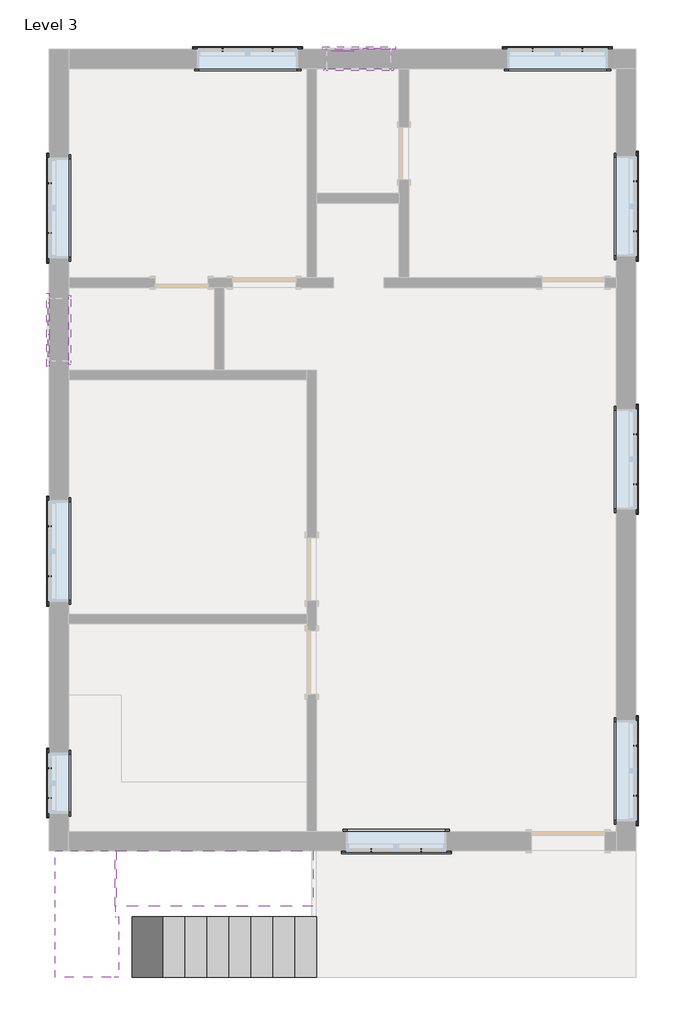
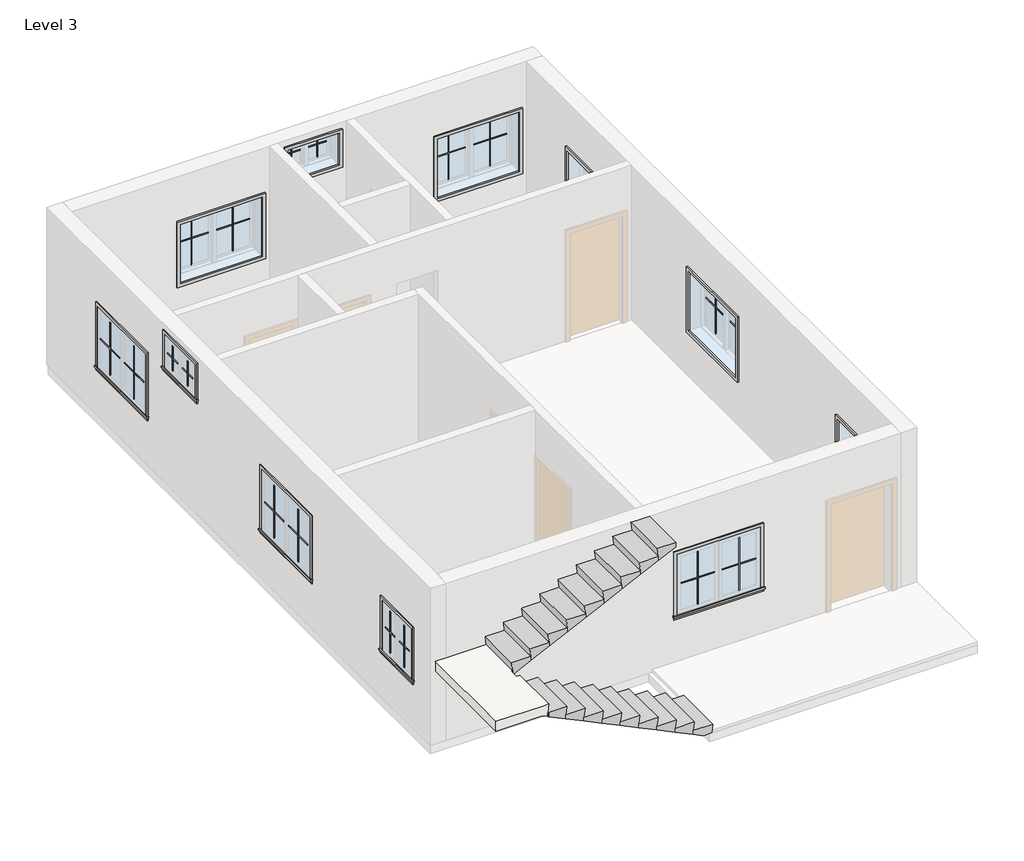
# One storey, part 2 of 2: 44 proxies, 2 stair flights, 1 slab.
"""IFC4 building model written with IfcOpenShell, lengths in millimetres."""

from ifc_helpers import new_model, si_unit, origin, place, context, project, spatial, faceted_brep, transform, mapped, element, save
from components import muntin_pattern_2x2_muntin_pattern_2x2_b3fe6957, muntin_pattern_2x2_muntin_pattern_2x2_3e0ecaf2, muntin_pattern_2x2_muntin_pattern_2x2_27d56209, muntin_pattern_2x2_muntin_pattern_2x2_bc89accc, muntin_pattern_2x2_muntin_pattern_2x2_1fe271a4, muntin_pattern_2x2_muntin_pattern_2x2_11ff06db, trim_window_exterior_flat_with_sill_41619996, trim_window_exterior_flat_with_sill_40e754a6, trim_window_exterior_flat_with_sill_f4abd27b, trim_window_interior_flat_picture_frame_51c85655, trim_window_interior_flat_picture_frame_6592d821, trim_window_interior_flat_picture_frame_286514af

model = new_model("IFC4")

# Units and contexts
model_context = context("Model", 3, world=origin())
ifc_project = project(units=[si_unit("LENGTHUNIT", "METRE", prefix="MILLI")], contexts=[model_context])

# Site, building, storey
site = spatial("IfcSite", under=ifc_project)
building = spatial("IfcBuilding", under=site)
storey = spatial("IfcBuildingStorey", under=building, Name="Level 3", Elevation=6096.0)

# Proxies
placement = place(None, origin())
muntin_pattern_2x2_muntin_pattern_2x2_shape = muntin_pattern_2x2_muntin_pattern_2x2_b3fe6957(model_context)
element("IfcBuildingElementProxy", 1, Name="Muntin Pattern_2x2 : Muntin Pattern_2x2", ObjectType="Muntin Pattern_2x2 : Muntin Pattern_2x2", at=placement, inside=storey, context=model_context, shape_type="MappedRepresentation", body=[
    mapped(muntin_pattern_2x2_muntin_pattern_2x2_shape, transform((-8839.6634077, -4303.4328663, 7080.25), x_axis=(0.0, 1.0, 0.0), y_axis=(-1.0, 0.0, 0.0), z_axis=(0.0, 0.0, 1.0))),
])
muntin_pattern_2x2_muntin_pattern_2x2_2_shape = muntin_pattern_2x2_muntin_pattern_2x2_3e0ecaf2(model_context)
element("IfcBuildingElementProxy", 2, Name="Muntin Pattern_2x2 : Muntin Pattern_2x2", ObjectType="Muntin Pattern_2x2 : Muntin Pattern_2x2", at=placement, inside=storey, context=model_context, shape_type="MappedRepresentation", body=[
    mapped(muntin_pattern_2x2_muntin_pattern_2x2_2_shape, transform((-8839.6634077, -3874.8078663, 7080.25), x_axis=(0.0, -1.0, 0.0), y_axis=(1.0, 0.0, 0.0), z_axis=(0.0, 0.0, 1.0))),
])
muntin_pattern_2x2_muntin_pattern_2x2_3_shape = muntin_pattern_2x2_muntin_pattern_2x2_27d56209(model_context)
element("IfcBuildingElementProxy", 3, Name="Muntin Pattern_2x2 : Muntin Pattern_2x2", ObjectType="Muntin Pattern_2x2 : Muntin Pattern_2x2", at=placement, inside=storey, context=model_context, shape_type="MappedRepresentation", body=[
    mapped(muntin_pattern_2x2_muntin_pattern_2x2_3_shape, transform((-8839.6634077, 2226.7657273, 8299.45), x_axis=(0.0, 1.0, 0.0), y_axis=(-1.0, 0.0, 0.0), z_axis=(0.0, 0.0, 1.0))),
])
element("IfcBuildingElementProxy", 4, Name="Muntin Pattern_2x2 : Muntin Pattern_2x2", ObjectType="Muntin Pattern_2x2 : Muntin Pattern_2x2", at=placement, inside=storey, context=model_context, shape_type="MappedRepresentation", body=[
    mapped(muntin_pattern_2x2_muntin_pattern_2x2_3_shape, transform((-4603.9220229, 6494.5392844, 8299.45), x_axis=(1.0, 0.0, 0.0), y_axis=(0.0, 1.0, 0.0), z_axis=(0.0, 0.0, 1.0))),
])
muntin_pattern_2x2_muntin_pattern_2x2_4_shape = muntin_pattern_2x2_muntin_pattern_2x2_bc89accc(model_context)
element("IfcBuildingElementProxy", 5, Name="Muntin Pattern_2x2 : Muntin Pattern_2x2", ObjectType="Muntin Pattern_2x2 : Muntin Pattern_2x2", at=placement, inside=storey, context=model_context, shape_type="MappedRepresentation", body=[
    mapped(muntin_pattern_2x2_muntin_pattern_2x2_4_shape, transform((-8839.6634077, 2680.7907273, 8299.45), x_axis=(0.0, -1.0, 0.0), y_axis=(1.0, 0.0, 0.0), z_axis=(0.0, 0.0, 1.0))),
])
element("IfcBuildingElementProxy", 6, Name="Muntin Pattern_2x2 : Muntin Pattern_2x2", ObjectType="Muntin Pattern_2x2 : Muntin Pattern_2x2", at=placement, inside=storey, context=model_context, shape_type="MappedRepresentation", body=[
    mapped(muntin_pattern_2x2_muntin_pattern_2x2_4_shape, transform((-4149.8970229, 6494.5392844, 8299.45), x_axis=(-1.0, 0.0, 0.0), y_axis=(0.0, -1.0, 0.0), z_axis=(0.0, 0.0, 1.0))),
])
muntin_pattern_2x2_muntin_pattern_2x2_5_shape = muntin_pattern_2x2_muntin_pattern_2x2_1fe271a4(model_context)
element("IfcBuildingElementProxy", 7, Name="Muntin Pattern_2x2 : Muntin Pattern_2x2", ObjectType="Muntin Pattern_2x2 : Muntin Pattern_2x2", at=placement, inside=storey, context=model_context, shape_type="MappedRepresentation", body=[
    mapped(muntin_pattern_2x2_muntin_pattern_2x2_5_shape, transform((-385.3035282, -3550.9578663, 7080.25), x_axis=(0.0, -1.0, 0.0), y_axis=(1.0, 0.0, 0.0), z_axis=(0.0, 0.0, 1.0))),
])
element("IfcBuildingElementProxy", 8, Name="Muntin Pattern_2x2 : Muntin Pattern_2x2", ObjectType="Muntin Pattern_2x2 : Muntin Pattern_2x2", at=placement, inside=storey, context=model_context, shape_type="MappedRepresentation", body=[
    mapped(muntin_pattern_2x2_muntin_pattern_2x2_5_shape, transform((-385.3035282, 944.8421337, 7080.25), x_axis=(0.0, -1.0, 0.0), y_axis=(1.0, 0.0, 0.0), z_axis=(0.0, 0.0, 1.0))),
])
element("IfcBuildingElementProxy", 9, Name="Muntin Pattern_2x2 : Muntin Pattern_2x2", ObjectType="Muntin Pattern_2x2 : Muntin Pattern_2x2", at=placement, inside=storey, context=model_context, shape_type="MappedRepresentation", body=[
    mapped(muntin_pattern_2x2_muntin_pattern_2x2_5_shape, transform((-385.3035282, 4597.1928819, 7080.25), x_axis=(0.0, -1.0, 0.0), y_axis=(1.0, 0.0, 0.0), z_axis=(0.0, 0.0, 1.0))),
])
element("IfcBuildingElementProxy", 10, Name="Muntin Pattern_2x2 : Muntin Pattern_2x2", ObjectType="Muntin Pattern_2x2 : Muntin Pattern_2x2", at=placement, inside=storey, context=model_context, shape_type="MappedRepresentation", body=[
    mapped(muntin_pattern_2x2_muntin_pattern_2x2_5_shape, transform((-1866.4410282, 6494.5392844, 7080.25), x_axis=(1.0, 0.0, 0.0), y_axis=(0.0, 1.0, 0.0), z_axis=(0.0, 0.0, 1.0))),
])
element("IfcBuildingElementProxy", 11, Name="Muntin Pattern_2x2 : Muntin Pattern_2x2", ObjectType="Muntin Pattern_2x2 : Muntin Pattern_2x2", at=placement, inside=storey, context=model_context, shape_type="MappedRepresentation", body=[
    mapped(muntin_pattern_2x2_muntin_pattern_2x2_5_shape, transform((-6342.5074828, 6494.5392844, 7080.25), x_axis=(1.0, 0.0, 0.0), y_axis=(0.0, 1.0, 0.0), z_axis=(0.0, 0.0, 1.0))),
])
element("IfcBuildingElementProxy", 12, Name="Muntin Pattern_2x2 : Muntin Pattern_2x2", ObjectType="Muntin Pattern_2x2 : Muntin Pattern_2x2", at=placement, inside=storey, context=model_context, shape_type="MappedRepresentation", body=[
    mapped(muntin_pattern_2x2_muntin_pattern_2x2_5_shape, transform((-8839.6634077, 3851.0678819, 7080.25), x_axis=(0.0, 1.0, 0.0), y_axis=(-1.0, 0.0, 0.0), z_axis=(0.0, 0.0, 1.0))),
])
element("IfcBuildingElementProxy", 13, Name="Muntin Pattern_2x2 : Muntin Pattern_2x2", ObjectType="Muntin Pattern_2x2 : Muntin Pattern_2x2", at=placement, inside=storey, context=model_context, shape_type="MappedRepresentation", body=[
    mapped(muntin_pattern_2x2_muntin_pattern_2x2_5_shape, transform((-8839.6634077, -1101.0873314, 7080.25), x_axis=(0.0, 1.0, 0.0), y_axis=(-1.0, 0.0, 0.0), z_axis=(0.0, 0.0, 1.0))),
])
element("IfcBuildingElementProxy", 14, Name="Muntin Pattern_2x2 : Muntin Pattern_2x2", ObjectType="Muntin Pattern_2x2 : Muntin Pattern_2x2", at=placement, inside=storey, context=model_context, shape_type="MappedRepresentation", body=[
    mapped(muntin_pattern_2x2_muntin_pattern_2x2_5_shape, transform((-3475.4824828, -5057.4953663, 7080.25), x_axis=(-1.0, 0.0, 0.0), y_axis=(0.0, -1.0, 0.0), z_axis=(0.0, 0.0, 1.0))),
])
muntin_pattern_2x2_muntin_pattern_2x2_6_shape = muntin_pattern_2x2_muntin_pattern_2x2_11ff06db(model_context)
element("IfcBuildingElementProxy", 15, Name="Muntin Pattern_2x2 : Muntin Pattern_2x2", ObjectType="Muntin Pattern_2x2 : Muntin Pattern_2x2", at=placement, inside=storey, context=model_context, shape_type="MappedRepresentation", body=[
    mapped(muntin_pattern_2x2_muntin_pattern_2x2_6_shape, transform((-385.3035282, -4271.6828663, 7080.25), x_axis=(0.0, 1.0, 0.0), y_axis=(-1.0, 0.0, 0.0), z_axis=(0.0, 0.0, 1.0))),
])
element("IfcBuildingElementProxy", 16, Name="Muntin Pattern_2x2 : Muntin Pattern_2x2", ObjectType="Muntin Pattern_2x2 : Muntin Pattern_2x2", at=placement, inside=storey, context=model_context, shape_type="MappedRepresentation", body=[
    mapped(muntin_pattern_2x2_muntin_pattern_2x2_6_shape, transform((-385.3035282, 224.1171337, 7080.25), x_axis=(0.0, 1.0, 0.0), y_axis=(-1.0, 0.0, 0.0), z_axis=(0.0, 0.0, 1.0))),
])
element("IfcBuildingElementProxy", 17, Name="Muntin Pattern_2x2 : Muntin Pattern_2x2", ObjectType="Muntin Pattern_2x2 : Muntin Pattern_2x2", at=placement, inside=storey, context=model_context, shape_type="MappedRepresentation", body=[
    mapped(muntin_pattern_2x2_muntin_pattern_2x2_6_shape, transform((-385.3035282, 3876.4678819, 7080.25), x_axis=(0.0, 1.0, 0.0), y_axis=(-1.0, 0.0, 0.0), z_axis=(0.0, 0.0, 1.0))),
])
element("IfcBuildingElementProxy", 18, Name="Muntin Pattern_2x2 : Muntin Pattern_2x2", ObjectType="Muntin Pattern_2x2 : Muntin Pattern_2x2", at=placement, inside=storey, context=model_context, shape_type="MappedRepresentation", body=[
    mapped(muntin_pattern_2x2_muntin_pattern_2x2_6_shape, transform((-1145.7160282, 6494.5392844, 7080.25), x_axis=(-1.0, 0.0, 0.0), y_axis=(0.0, -1.0, 0.0), z_axis=(0.0, 0.0, 1.0))),
])
element("IfcBuildingElementProxy", 19, Name="Muntin Pattern_2x2 : Muntin Pattern_2x2", ObjectType="Muntin Pattern_2x2 : Muntin Pattern_2x2", at=placement, inside=storey, context=model_context, shape_type="MappedRepresentation", body=[
    mapped(muntin_pattern_2x2_muntin_pattern_2x2_6_shape, transform((-5621.7824828, 6494.5392844, 7080.25), x_axis=(-1.0, 0.0, 0.0), y_axis=(0.0, -1.0, 0.0), z_axis=(0.0, 0.0, 1.0))),
])
element("IfcBuildingElementProxy", 20, Name="Muntin Pattern_2x2 : Muntin Pattern_2x2", ObjectType="Muntin Pattern_2x2 : Muntin Pattern_2x2", at=placement, inside=storey, context=model_context, shape_type="MappedRepresentation", body=[
    mapped(muntin_pattern_2x2_muntin_pattern_2x2_6_shape, transform((-8839.6634077, 4571.7928819, 7080.25), x_axis=(0.0, -1.0, 0.0), y_axis=(1.0, 0.0, 0.0), z_axis=(0.0, 0.0, 1.0))),
])
element("IfcBuildingElementProxy", 21, Name="Muntin Pattern_2x2 : Muntin Pattern_2x2", ObjectType="Muntin Pattern_2x2 : Muntin Pattern_2x2", at=placement, inside=storey, context=model_context, shape_type="MappedRepresentation", body=[
    mapped(muntin_pattern_2x2_muntin_pattern_2x2_6_shape, transform((-8839.6634077, -380.3623314, 7080.25), x_axis=(0.0, -1.0, 0.0), y_axis=(1.0, 0.0, 0.0), z_axis=(0.0, 0.0, 1.0))),
])
element("IfcBuildingElementProxy", 22, Name="Muntin Pattern_2x2 : Muntin Pattern_2x2", ObjectType="Muntin Pattern_2x2 : Muntin Pattern_2x2", at=placement, inside=storey, context=model_context, shape_type="MappedRepresentation", body=[
    mapped(muntin_pattern_2x2_muntin_pattern_2x2_6_shape, transform((-4196.2074828, -5057.4953663, 7080.25), x_axis=(1.0, 0.0, 0.0), y_axis=(0.0, 1.0, 0.0), z_axis=(0.0, 0.0, 1.0))),
])
trim_window_exterior_flat_with_sill_shape = trim_window_exterior_flat_with_sill_41619996(model_context)
element("IfcBuildingElementProxy", 23, Name="Trim-Window-Exterior-Flat : with Sill", ObjectType="Trim-Window-Exterior-Flat : with Sill", at=placement, inside=storey, context=model_context, shape_type="MappedRepresentation", body=[
    mapped(trim_window_exterior_flat_with_sill_shape, transform((-8849.1884077, -4089.1203663, 7924.8), x_axis=(0.0, -1.0, 0.0), y_axis=(0.0, 0.0, 1.0), z_axis=(-1.0, 0.0, 0.0))),
])
trim_window_exterior_flat_with_sill_2_shape = trim_window_exterior_flat_with_sill_40e754a6(model_context)
element("IfcBuildingElementProxy", 24, Name="Trim-Window-Exterior-Flat : with Sill", ObjectType="Trim-Window-Exterior-Flat : with Sill", at=placement, inside=storey, context=model_context, shape_type="MappedRepresentation", body=[
    mapped(trim_window_exterior_flat_with_sill_2_shape, transform((-8849.1884077, 2453.7782273, 8839.2), x_axis=(0.0, -1.0, 0.0), y_axis=(0.0, 0.0, 1.0), z_axis=(-1.0, 0.0, 0.0))),
])
element("IfcBuildingElementProxy", 25, Name="Trim-Window-Exterior-Flat : with Sill", ObjectType="Trim-Window-Exterior-Flat : with Sill", at=placement, inside=storey, context=model_context, shape_type="MappedRepresentation", body=[
    mapped(trim_window_exterior_flat_with_sill_2_shape, transform((-4376.9095229, 6504.0642844, 8839.2), x_axis=(-1.0, 0.0, 0.0), y_axis=(0.0, 0.0, 1.0), z_axis=(0.0, 1.0, 0.0))),
])
trim_window_exterior_flat_with_sill_3_shape = trim_window_exterior_flat_with_sill_f4abd27b(model_context)
element("IfcBuildingElementProxy", 26, Name="Trim-Window-Exterior-Flat : with Sill", ObjectType="Trim-Window-Exterior-Flat : with Sill", at=placement, inside=storey, context=model_context, shape_type="MappedRepresentation", body=[
    mapped(trim_window_exterior_flat_with_sill_3_shape, transform((-375.7785282, -3911.3203663, 8128.0), x_axis=(0.0, 1.0, 0.0), y_axis=(0.0, 0.0, 1.0), z_axis=(1.0, 0.0, 0.0))),
])
element("IfcBuildingElementProxy", 27, Name="Trim-Window-Exterior-Flat : with Sill", ObjectType="Trim-Window-Exterior-Flat : with Sill", at=placement, inside=storey, context=model_context, shape_type="MappedRepresentation", body=[
    mapped(trim_window_exterior_flat_with_sill_3_shape, transform((-375.7785282, 584.4796337, 8128.0), x_axis=(0.0, 1.0, 0.0), y_axis=(0.0, 0.0, 1.0), z_axis=(1.0, 0.0, 0.0))),
])
element("IfcBuildingElementProxy", 28, Name="Trim-Window-Exterior-Flat : with Sill", ObjectType="Trim-Window-Exterior-Flat : with Sill", at=placement, inside=storey, context=model_context, shape_type="MappedRepresentation", body=[
    mapped(trim_window_exterior_flat_with_sill_3_shape, transform((-375.7785282, 4236.8303819, 8128.0), x_axis=(0.0, 1.0, 0.0), y_axis=(0.0, 0.0, 1.0), z_axis=(1.0, 0.0, 0.0))),
])
element("IfcBuildingElementProxy", 29, Name="Trim-Window-Exterior-Flat : with Sill", ObjectType="Trim-Window-Exterior-Flat : with Sill", at=placement, inside=storey, context=model_context, shape_type="MappedRepresentation", body=[
    mapped(trim_window_exterior_flat_with_sill_3_shape, transform((-1506.0785282, 6504.0642844, 8128.0), x_axis=(-1.0, 0.0, 0.0), y_axis=(0.0, 0.0, 1.0), z_axis=(0.0, 1.0, 0.0))),
])
element("IfcBuildingElementProxy", 30, Name="Trim-Window-Exterior-Flat : with Sill", ObjectType="Trim-Window-Exterior-Flat : with Sill", at=placement, inside=storey, context=model_context, shape_type="MappedRepresentation", body=[
    mapped(trim_window_exterior_flat_with_sill_3_shape, transform((-5982.1449828, 6504.0642844, 8128.0), x_axis=(-1.0, 0.0, 0.0), y_axis=(0.0, 0.0, 1.0), z_axis=(0.0, 1.0, 0.0))),
])
element("IfcBuildingElementProxy", 31, Name="Trim-Window-Exterior-Flat : with Sill", ObjectType="Trim-Window-Exterior-Flat : with Sill", at=placement, inside=storey, context=model_context, shape_type="MappedRepresentation", body=[
    mapped(trim_window_exterior_flat_with_sill_3_shape, transform((-8849.1884077, 4211.4303819, 8128.0), x_axis=(0.0, -1.0, 0.0), y_axis=(0.0, 0.0, 1.0), z_axis=(-1.0, 0.0, 0.0))),
])
element("IfcBuildingElementProxy", 32, Name="Trim-Window-Exterior-Flat : with Sill", ObjectType="Trim-Window-Exterior-Flat : with Sill", at=placement, inside=storey, context=model_context, shape_type="MappedRepresentation", body=[
    mapped(trim_window_exterior_flat_with_sill_3_shape, transform((-8849.1884077, -740.7248314, 8128.0), x_axis=(0.0, -1.0, 0.0), y_axis=(0.0, 0.0, 1.0), z_axis=(-1.0, 0.0, 0.0))),
])
element("IfcBuildingElementProxy", 33, Name="Trim-Window-Exterior-Flat : with Sill", ObjectType="Trim-Window-Exterior-Flat : with Sill", at=placement, inside=storey, context=model_context, shape_type="MappedRepresentation", body=[
    mapped(trim_window_exterior_flat_with_sill_3_shape, transform((-3835.8449828, -5067.0203663, 8128.0), x_axis=(1.0, 0.0, 0.0), y_axis=(0.0, 0.0, 1.0), z_axis=(0.0, -1.0, 0.0))),
])
trim_window_interior_flat_picture_frame_shape = trim_window_interior_flat_picture_frame_51c85655(model_context)
element("IfcBuildingElementProxy", 34, Name="Trim-Window-Interior-Flat : Picture Frame", ObjectType="Trim-Window-Interior-Flat : Picture Frame", at=placement, inside=storey, context=model_context, shape_type="MappedRepresentation", body=[
    mapped(trim_window_interior_flat_picture_frame_shape, transform((-8569.7884077, -4089.1203663, 7924.8), x_axis=(0.0, 1.0, 0.0), y_axis=(0.0, 0.0, 1.0), z_axis=(1.0, 0.0, 0.0))),
])
trim_window_interior_flat_picture_frame_2_shape = trim_window_interior_flat_picture_frame_6592d821(model_context)
element("IfcBuildingElementProxy", 35, Name="Trim-Window-Interior-Flat : Picture Frame", ObjectType="Trim-Window-Interior-Flat : Picture Frame", at=placement, inside=storey, context=model_context, shape_type="MappedRepresentation", body=[
    mapped(trim_window_interior_flat_picture_frame_2_shape, transform((-8569.7884077, 2453.7782273, 8839.2), x_axis=(0.0, 1.0, 0.0), y_axis=(0.0, 0.0, 1.0), z_axis=(1.0, 0.0, 0.0))),
])
element("IfcBuildingElementProxy", 36, Name="Trim-Window-Interior-Flat : Picture Frame", ObjectType="Trim-Window-Interior-Flat : Picture Frame", at=placement, inside=storey, context=model_context, shape_type="MappedRepresentation", body=[
    mapped(trim_window_interior_flat_picture_frame_2_shape, transform((-4376.9095229, 6224.6642844, 8839.2), x_axis=(1.0, 0.0, 0.0), y_axis=(0.0, 0.0, 1.0), z_axis=(0.0, -1.0, 0.0))),
])
trim_window_interior_flat_picture_frame_3_shape = trim_window_interior_flat_picture_frame_286514af(model_context)
element("IfcBuildingElementProxy", 37, Name="Trim-Window-Interior-Flat : Picture Frame", ObjectType="Trim-Window-Interior-Flat : Picture Frame", at=placement, inside=storey, context=model_context, shape_type="MappedRepresentation", body=[
    mapped(trim_window_interior_flat_picture_frame_3_shape, transform((-655.1785282, -3911.3203663, 8128.0), x_axis=(0.0, -1.0, 0.0), y_axis=(0.0, 0.0, 1.0), z_axis=(-1.0, 0.0, 0.0))),
])
element("IfcBuildingElementProxy", 38, Name="Trim-Window-Interior-Flat : Picture Frame", ObjectType="Trim-Window-Interior-Flat : Picture Frame", at=placement, inside=storey, context=model_context, shape_type="MappedRepresentation", body=[
    mapped(trim_window_interior_flat_picture_frame_3_shape, transform((-655.1785282, 584.4796337, 8128.0), x_axis=(0.0, -1.0, 0.0), y_axis=(0.0, 0.0, 1.0), z_axis=(-1.0, 0.0, 0.0))),
])
element("IfcBuildingElementProxy", 39, Name="Trim-Window-Interior-Flat : Picture Frame", ObjectType="Trim-Window-Interior-Flat : Picture Frame", at=placement, inside=storey, context=model_context, shape_type="MappedRepresentation", body=[
    mapped(trim_window_interior_flat_picture_frame_3_shape, transform((-655.1785282, 4236.8303819, 8128.0), x_axis=(0.0, -1.0, 0.0), y_axis=(0.0, 0.0, 1.0), z_axis=(-1.0, 0.0, 0.0))),
])
element("IfcBuildingElementProxy", 40, Name="Trim-Window-Interior-Flat : Picture Frame", ObjectType="Trim-Window-Interior-Flat : Picture Frame", at=placement, inside=storey, context=model_context, shape_type="MappedRepresentation", body=[
    mapped(trim_window_interior_flat_picture_frame_3_shape, transform((-1506.0785282, 6224.6642844, 8128.0), x_axis=(1.0, 0.0, 0.0), y_axis=(0.0, 0.0, 1.0), z_axis=(0.0, -1.0, 0.0))),
])
element("IfcBuildingElementProxy", 41, Name="Trim-Window-Interior-Flat : Picture Frame", ObjectType="Trim-Window-Interior-Flat : Picture Frame", at=placement, inside=storey, context=model_context, shape_type="MappedRepresentation", body=[
    mapped(trim_window_interior_flat_picture_frame_3_shape, transform((-5982.1449828, 6224.6642844, 8128.0), x_axis=(1.0, 0.0, 0.0), y_axis=(0.0, 0.0, 1.0), z_axis=(0.0, -1.0, 0.0))),
])
element("IfcBuildingElementProxy", 42, Name="Trim-Window-Interior-Flat : Picture Frame", ObjectType="Trim-Window-Interior-Flat : Picture Frame", at=placement, inside=storey, context=model_context, shape_type="MappedRepresentation", body=[
    mapped(trim_window_interior_flat_picture_frame_3_shape, transform((-8569.7884077, 4211.4303819, 8128.0), x_axis=(0.0, 1.0, 0.0), y_axis=(0.0, 0.0, 1.0), z_axis=(1.0, 0.0, 0.0))),
])
element("IfcBuildingElementProxy", 43, Name="Trim-Window-Interior-Flat : Picture Frame", ObjectType="Trim-Window-Interior-Flat : Picture Frame", at=placement, inside=storey, context=model_context, shape_type="MappedRepresentation", body=[
    mapped(trim_window_interior_flat_picture_frame_3_shape, transform((-8569.7884077, -740.7248314, 8128.0), x_axis=(0.0, 1.0, 0.0), y_axis=(0.0, 0.0, 1.0), z_axis=(1.0, 0.0, 0.0))),
])
element("IfcBuildingElementProxy", 44, Name="Trim-Window-Interior-Flat : Picture Frame", ObjectType="Trim-Window-Interior-Flat : Picture Frame", at=placement, inside=storey, context=model_context, shape_type="MappedRepresentation", body=[
    mapped(trim_window_interior_flat_picture_frame_3_shape, transform((-3835.8449828, -4787.6203663, 8128.0), x_axis=(-1.0, 0.0, 0.0), y_axis=(0.0, 0.0, 1.0), z_axis=(0.0, 1.0, 0.0))),
])

# Slab
element("IfcSlab", 45, ObjectType="7\" Thickness", at=placement, inside=storey, context=model_context, shape_type="Brep", body=[
    faceted_brep([(-7896.6884077, -6018.2039507, 7620.0), (-7896.6884077, -5868.2058051, 7620.0), (-7877.6384077, -5868.2058051, 7620.0), (-7877.6384077, -5067.0203663, 7620.0), (-7896.6884077, -5067.0203663, 7620.0), (-8101.3126638, -5067.0203663, 7620.0), (-8760.2884077, -5067.0203663, 7620.0), (-8760.2884077, -6894.0922127, 7620.0), (-7955.5707267, -6894.0922127, 7620.0), (-7842.6949828, -6894.0922127, 7620.0), (-7842.6949828, -6018.2039507, 7620.0), (-7861.7449828, -6018.2039507, 7467.6), (-7861.7449828, -6894.0922127, 7467.6), (-7861.7449828, -6894.0922127, 7397.1636429), (-7861.7449828, -6018.2039507, 7397.1636429), (-7955.5707267, -6018.2039507, 7442.2), (-7896.6884077, -6018.2039507, 7442.2), (-7896.6884077, -5868.2058051, 7442.2), (-7896.6884077, -5868.2058051, 7540.4196429), (-7877.6384077, -5868.2058051, 7549.5636429), (-7877.6384077, -5067.0203663, 7549.5636429), (-7896.6884077, -5067.0203663, 7540.4196429), (-8101.3126638, -5067.0203663, 7442.2), (-8760.2884077, -5067.0203663, 7442.2), (-8760.2884077, -6894.0922127, 7442.2), (-7955.5707267, -6894.0922127, 7442.2), (-8101.3126638, -5868.2058051, 7442.2)], [[[0, 1, 2, 3, 4, 5, 6, 7, 8, 9, 10]], [[11, 12, 13, 14]], [[0, 10, 11, 14, 15, 16]], [[1, 0, 16, 17, 18]], [[2, 1, 18, 19]], [[3, 2, 19, 20]], [[4, 3, 20, 21]], [[4, 21, 22, 23, 6, 5]], [[7, 6, 23, 24]], [[12, 9, 8, 7, 24, 25, 13]], [[10, 9, 12, 11]], [[26, 17, 16, 15, 25, 24, 23, 22]], [[17, 26, 18]], [[25, 15, 14, 13]], [[26, 22, 21, 20, 19, 18]]]),
])

# Stair flights
element("IfcStairFlight", 46, ObjectType="3/4\" Nosing", at=placement, inside=storey, context=model_context, shape_type="Brep", body=[
    faceted_brep([(-4985.1949828, -6894.0922127, 6248.4), (-4985.1949828, -6018.2039507, 6248.4), (-5321.7449828, -6018.2039507, 6248.4), (-5321.7449828, -6894.0922127, 6248.4), (-5321.7449828, -6894.0922127, 6177.9636429), (-5150.9873934, -6894.0922127, 6096.0), (-5004.2449828, -6894.0922127, 6096.0), (-5004.2449828, -6018.2039507, 6096.0), (-5150.9873934, -6018.2039507, 6096.0), (-5321.7449828, -6018.2039507, 6177.9636429), (-5302.6949828, -6894.0922127, 6400.8), (-5302.6949828, -6018.2039507, 6400.8), (-5639.2449828, -6018.2039507, 6400.8), (-5639.2449828, -6894.0922127, 6400.8), (-5639.2449828, -6894.0922127, 6330.3636429), (-5639.2449828, -6018.2039507, 6330.3636429), (-5620.1949828, -6894.0922127, 6553.2), (-5620.1949828, -6018.2039507, 6553.2), (-5956.7449828, -6018.2039507, 6553.2), (-5956.7449828, -6894.0922127, 6553.2), (-5956.7449828, -6894.0922127, 6482.7636429), (-5956.7449828, -6018.2039507, 6482.7636429), (-5937.6949828, -6894.0922127, 6705.6), (-5937.6949828, -6018.2039507, 6705.6), (-6274.2449828, -6018.2039507, 6705.6), (-6274.2449828, -6894.0922127, 6705.6), (-6274.2449828, -6894.0922127, 6635.1636429), (-6274.2449828, -6018.2039507, 6635.1636429), (-6255.1949828, -6894.0922127, 6858.0), (-6255.1949828, -6018.2039507, 6858.0), (-6591.7449828, -6018.2039507, 6858.0), (-6591.7449828, -6894.0922127, 6858.0), (-6591.7449828, -6894.0922127, 6787.5636429), (-6591.7449828, -6018.2039507, 6787.5636429), (-6572.6949828, -6894.0922127, 7010.4), (-6572.6949828, -6018.2039507, 7010.4), (-6909.2449828, -6018.2039507, 7010.4), (-6909.2449828, -6894.0922127, 7010.4), (-6909.2449828, -6894.0922127, 6939.9636429), (-6909.2449828, -6018.2039507, 6939.9636429), (-6890.1949828, -6894.0922127, 7162.8), (-6890.1949828, -6018.2039507, 7162.8), (-7226.7449828, -6018.2039507, 7162.8), (-7226.7449828, -6894.0922127, 7162.8), (-7226.7449828, -6894.0922127, 7092.3636429), (-7226.7449828, -6018.2039507, 7092.3636429), (-7207.6949828, -6894.0922127, 7315.2), (-7207.6949828, -6018.2039507, 7315.2), (-7544.2449828, -6018.2039507, 7315.2), (-7544.2449828, -6894.0922127, 7315.2), (-7544.2449828, -6894.0922127, 7244.7636429), (-7544.2449828, -6018.2039507, 7244.7636429), (-7861.7449828, -6894.0922127, 7467.6), (-7842.6949828, -6894.0922127, 7467.6), (-7525.1949828, -6894.0922127, 7467.6), (-7525.1949828, -6018.2039507, 7467.6), (-7842.6949828, -6018.2039507, 7467.6), (-7861.7449828, -6018.2039507, 7467.6), (-7861.7449828, -6894.0922127, 7397.1636429), (-7842.6949828, -6894.0922127, 7388.0196429), (-7842.6949828, -6018.2039507, 7388.0196429), (-7861.7449828, -6018.2039507, 7397.1636429)], [[[0, 1, 2, 3]], [[0, 3, 4, 5, 6]], [[2, 1, 7, 8, 9]], [[10, 11, 12, 13]], [[10, 13, 14, 4, 3]], [[12, 11, 2, 9, 15]], [[16, 17, 18, 19]], [[16, 19, 20, 14, 13]], [[18, 17, 12, 15, 21]], [[22, 23, 24, 25]], [[22, 25, 26, 20, 19]], [[24, 23, 18, 21, 27]], [[28, 29, 30, 31]], [[28, 31, 32, 26, 25]], [[30, 29, 24, 27, 33]], [[34, 35, 36, 37]], [[34, 37, 38, 32, 31]], [[36, 35, 30, 33, 39]], [[40, 41, 42, 43]], [[40, 43, 44, 38, 37]], [[42, 41, 36, 39, 45]], [[46, 47, 48, 49]], [[46, 49, 50, 44, 43]], [[48, 47, 42, 45, 51]], [[52, 53, 54, 55, 56, 57]], [[53, 52, 58, 59]], [[54, 53, 59, 50, 49]], [[56, 55, 48, 51, 60]], [[57, 56, 60, 61]], [[52, 57, 61, 58]], [[1, 0, 6, 7]], [[3, 2, 11, 10]], [[13, 12, 17, 16]], [[19, 18, 23, 22]], [[25, 24, 29, 28]], [[31, 30, 35, 34]], [[37, 36, 41, 40]], [[43, 42, 47, 46]], [[49, 48, 55, 54]], [[7, 6, 5, 8]], [[8, 5, 4, 14, 20, 26, 32, 38, 44, 50, 59, 58, 61, 60, 51, 45, 39, 33, 27, 21, 15, 9]]]),
])
element("IfcStairFlight", 47, ObjectType="3/4\" Nosing", at=placement, inside=storey, context=model_context, shape_type="Brep", body=[
    faceted_brep([(-7896.6884077, -5067.0203663, 7772.4), (-7896.6884077, -5868.2058051, 7772.4), (-7560.1384077, -5868.2058051, 7772.4), (-7560.1384077, -5067.0203663, 7772.4), (-7560.1384077, -5067.0203663, 7701.9636429), (-7877.6384077, -5067.0203663, 7549.5636429), (-7877.6384077, -5067.0203663, 7620.0), (-7877.6384077, -5868.2058051, 7620.0), (-7877.6384077, -5868.2058051, 7549.5636429), (-7560.1384077, -5868.2058051, 7701.9636429), (-7579.1884077, -5067.0203663, 7924.8), (-7579.1884077, -5868.2058051, 7924.8), (-7242.6384077, -5868.2058051, 7924.8), (-7242.6384077, -5067.0203663, 7924.8), (-7242.6384077, -5067.0203663, 7854.3636429), (-7242.6384077, -5868.2058051, 7854.3636429), (-7261.6884077, -5067.0203663, 8077.2), (-7261.6884077, -5868.2058051, 8077.2), (-6925.1384077, -5868.2058051, 8077.2), (-6925.1384077, -5067.0203663, 8077.2), (-6925.1384077, -5067.0203663, 8006.7636429), (-6925.1384077, -5868.2058051, 8006.7636429), (-6944.1884077, -5067.0203663, 8229.6), (-6944.1884077, -5868.2058051, 8229.6), (-6607.6384077, -5868.2058051, 8229.6), (-6607.6384077, -5067.0203663, 8229.6), (-6607.6384077, -5067.0203663, 8159.1636429), (-6607.6384077, -5868.2058051, 8159.1636429), (-6626.6884077, -5067.0203663, 8382.0), (-6626.6884077, -5868.2058051, 8382.0), (-6290.1384077, -5868.2058051, 8382.0), (-6290.1384077, -5067.0203663, 8382.0), (-6290.1384077, -5067.0203663, 8311.5636429), (-6290.1384077, -5868.2058051, 8311.5636429), (-6309.1884077, -5067.0203663, 8534.4), (-6309.1884077, -5868.2058051, 8534.4), (-5972.6384077, -5868.2058051, 8534.4), (-5972.6384077, -5067.0203663, 8534.4), (-5972.6384077, -5067.0203663, 8463.9636429), (-5972.6384077, -5868.2058051, 8463.9636429), (-5991.6884077, -5067.0203663, 8686.8), (-5991.6884077, -5868.2058051, 8686.8), (-5655.1384077, -5868.2058051, 8686.8), (-5655.1384077, -5067.0203663, 8686.8), (-5655.1384077, -5067.0203663, 8616.3636429), (-5655.1384077, -5868.2058051, 8616.3636429), (-5674.1884077, -5067.0203663, 8839.2), (-5674.1884077, -5868.2058051, 8839.2), (-5337.6384077, -5868.2058051, 8839.2), (-5337.6384077, -5067.0203663, 8839.2), (-5337.6384077, -5067.0203663, 8768.7636429), (-5337.6384077, -5868.2058051, 8768.7636429), (-5356.6884077, -5067.0203663, 8991.6), (-5356.6884077, -5868.2058051, 8991.6), (-5039.1884077, -5868.2058051, 8991.6), (-5039.1884077, -5067.0203663, 8991.6), (-5039.1884077, -5067.0203663, 8912.0196429), (-5039.1884077, -5868.2058051, 8912.0196429)], [[[0, 1, 2, 3]], [[0, 3, 4, 5, 6]], [[7, 6, 5, 8]], [[2, 1, 7, 8, 9]], [[10, 11, 12, 13]], [[10, 13, 14, 4, 3]], [[12, 11, 2, 9, 15]], [[16, 17, 18, 19]], [[16, 19, 20, 14, 13]], [[18, 17, 12, 15, 21]], [[22, 23, 24, 25]], [[22, 25, 26, 20, 19]], [[24, 23, 18, 21, 27]], [[28, 29, 30, 31]], [[28, 31, 32, 26, 25]], [[30, 29, 24, 27, 33]], [[34, 35, 36, 37]], [[34, 37, 38, 32, 31]], [[36, 35, 30, 33, 39]], [[40, 41, 42, 43]], [[40, 43, 44, 38, 37]], [[42, 41, 36, 39, 45]], [[46, 47, 48, 49]], [[46, 49, 50, 44, 43]], [[48, 47, 42, 45, 51]], [[1, 0, 6, 7]], [[11, 10, 3, 2]], [[17, 16, 13, 12]], [[23, 22, 19, 18]], [[29, 28, 25, 24]], [[35, 34, 31, 30]], [[41, 40, 37, 36]], [[47, 46, 43, 42]], [[52, 53, 54, 55]], [[52, 55, 56, 50, 49]], [[54, 53, 48, 51, 57]], [[55, 54, 57, 56]], [[53, 52, 49, 48]], [[5, 4, 14, 20, 26, 32, 38, 44, 50, 56, 57, 51, 45, 39, 33, 27, 21, 15, 9, 8]]]),
])

save(model, "model.ifc")

# Revit data of these elements
# Type "Muntin Pattern_2x2 : Muntin Pattern_2x2"
#   Width [instance default] = 48"
#   Thickness = 0.5"
#   Height [instance default] = 48"
#   Distance = 0.75"
#   Interior Material [instance default] = none
#   Exterior Material [instance default] = none
#   Default Elevation = 0
# Type "Trim-Window-Exterior-Flat : with Sill"
#   Trim Width = 2.25"
#   Trim Thickness_Picture Frame = 1.25"
#   Trim Thickness_with Sill = 0.75"
#   Sill Thickness = 1.25"
#   Opening Width [instance default] = 24"
#   Opening Height [instance default] = 36"
#   Default Elevation = 48"
#   Sill = yes
#   Picture Frame = no
#   Trim Material [instance default] = none
# Type "Trim-Window-Interior-Flat : Picture Frame"
#   Trim Thickness_Picture Frame = 1.25"
#   Trim Width = 2.25"
#   Trim Thickness_with Sill = 0.75"
#   Sill Thickness = 1.25"
#   Opening Width [instance default] = 24"
#   Opening Height [instance default] = 36"
#   Default Elevation = 48"
#   Sill = no
#   Picture Frame = yes
#   Trim Material [instance default] = none
# Elements 1, 2 (IfcBuildingElementProxy, "Muntin Pattern_2x2 : Muntin Pattern_2x2")
#   Width = 11.625"
#   Height = 30.5"
#   Interior Material = Wood - Stained
#   Exterior Material = Clad - White
#   Phase Created = New Construction
#   Materials on its faces: "Clad - White", "Wood - Stained"
# Elements 3, 4, 5, 6 (IfcBuildingElementProxy, "Muntin Pattern_2x2 : Muntin Pattern_2x2")
#   Width = 12.625"
#   Height = 18.5"
#   Interior Material = Wood - Stained
#   Exterior Material = Clad - White
#   Phase Created = New Construction
#   Materials on its faces: "Clad - White", "Wood - Stained"
# Elements 7, 8, 9, 10, 11, 12, 13, 14, 15, 16, 17, 18, 19, 20, 21, 22 (IfcBuildingElementProxy, "Muntin Pattern_2x2 : Muntin Pattern_2x2")
#   Width = 23.125"
#   Height = 38.5"
#   Interior Material = Wood - Stained
#   Exterior Material = Clad - White
#   Phase Created = New Construction
#   Materials on its faces: "Clad - White", "Wood - Stained"
# Element 23 (IfcBuildingElementProxy, "Trim-Window-Exterior-Flat : with Sill")
#   Opening Width = 34"
#   Opening Height = 36"
#   Trim Material = Clad - White
#   Phase Created = New Construction
#   Materials on its faces: "Clad - White"
# Elements 24, 25 (IfcBuildingElementProxy, "Trim-Window-Exterior-Flat : with Sill")
#   Opening Width = 36"
#   Opening Height = 24"
#   Trim Material = Clad - White
#   Phase Created = New Construction
#   Materials on its faces: "Clad - White"
# Elements 26, 27, 28, 29, 30, 31, 32, 33 (IfcBuildingElementProxy, "Trim-Window-Exterior-Flat : with Sill")
#   Opening Width = 57"
#   Opening Height = 44"
#   Trim Material = Clad - White
#   Phase Created = New Construction
#   Materials on its faces: "Clad - White"
# Element 34 (IfcBuildingElementProxy, "Trim-Window-Interior-Flat : Picture Frame")
#   Opening Width = 34"
#   Opening Height = 36"
#   Trim Material = Wood - Stained
#   Phase Created = New Construction
#   Materials on its faces: "Wood - Stained"
# Elements 35, 36 (IfcBuildingElementProxy, "Trim-Window-Interior-Flat : Picture Frame")
#   Opening Width = 36"
#   Opening Height = 24"
#   Trim Material = Wood - Stained
#   Phase Created = New Construction
#   Materials on its faces: "Wood - Stained"
# Elements 37, 38, 39, 40, 41, 42, 43, 44 (IfcBuildingElementProxy, "Trim-Window-Interior-Flat : Picture Frame")
#   Opening Width = 57"
#   Opening Height = 44"
#   Trim Material = Wood - Stained
#   Phase Created = New Construction
#   Materials on its faces: "Wood - Stained"
# Element 45 (IfcSlab, "7\" Thickness")
#   Phase Created = New Construction
#   Materials on its faces: "Concrete, Cast-in-Place gray"
# Elements 46, 47 (IfcStairFlight, "3/4\" Nosing")
#   Phase Created = New Construction
#   Materials on its faces: "Concrete, Cast-in-Place gray"
# Materials
#   "Clad - White": class "Wood", colour RGB 242 242 238, transparency 0, Cost = 0
#   "Wood - Stained": class "Wood", colour RGB 224 178 126, transparency 0, Cost = 0
#   "Concrete, Cast-in-Place gray": class "Concrete", colour RGB 192 192 192, transparency 0, Description = "Cast-in-place concrete", Cost = 0
